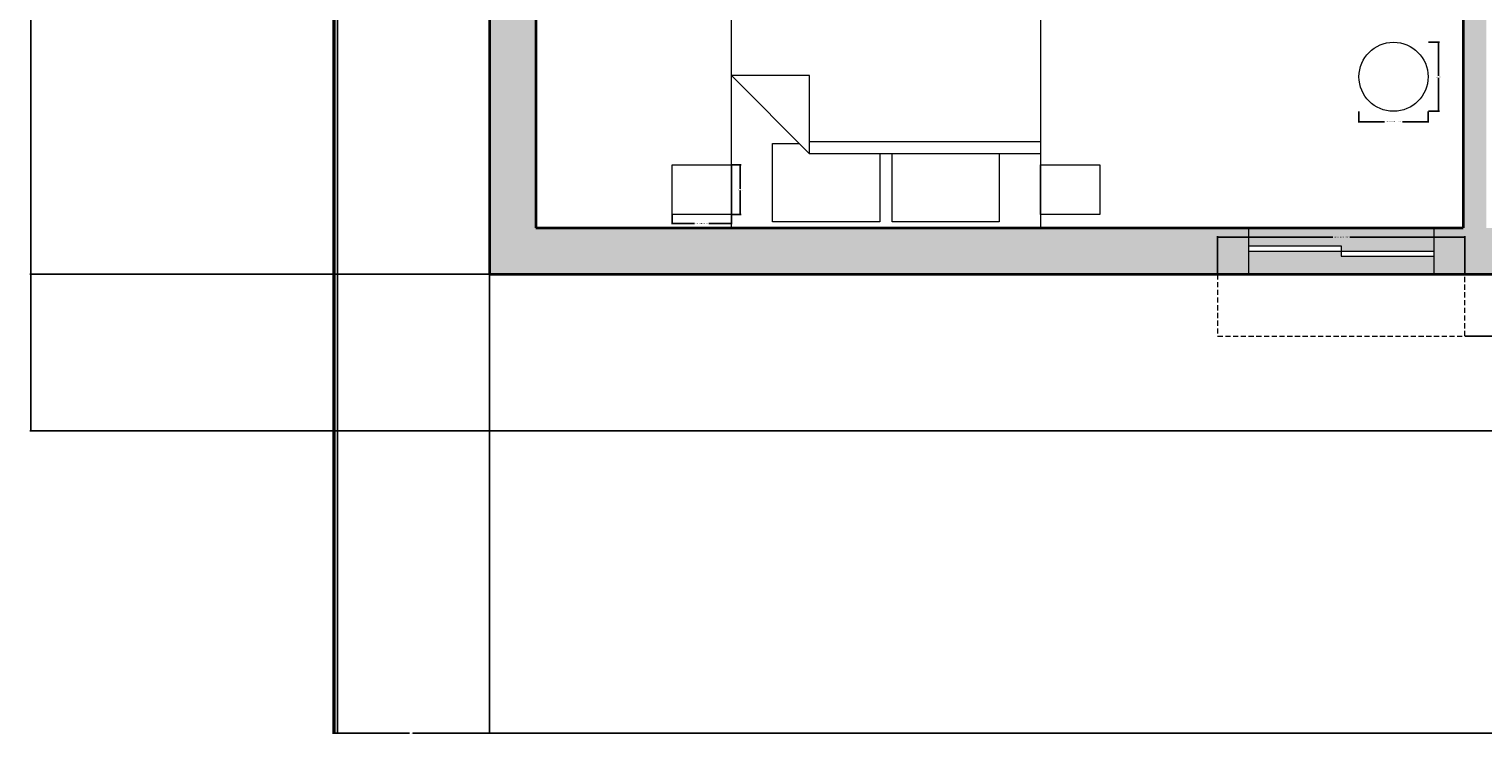
# Model space of a CAD drawing. Units: inches. Extents: x 1693 to 2974, y 2201 to 2965.
# Tile 1 of 24: x 1693 to 1976, y 2201 to 2337. Entities that reach past the tile are written whole.
import ezdxf

# ---------------------------------------------------------------- set-up
doc = ezdxf.new("R2010")
doc.units = ezdxf.units.IN
doc.header["$LTSCALE"] = 2
doc.header["$MEASUREMENT"] = 0
doc.linetypes.add('HIDDEN', pattern=[0.375, 0.25, -0.125])
for name, color, linetype, lineweight in [('A-ANNO-DIMS', 2, 'Continuous', 18), ('A-FURN', 8, 'Continuous', 18), ('A-GLAZ', 4, 'Continuous', 18), ('A-GLAZ-OVHD', 8, 'HIDDEN', 13), ('A-WALL', 7, 'Continuous', 35)]:
    doc.layers.add(name, color=color, linetype=linetype, lineweight=lineweight)
doc.layers.add('A-GLAZ-PATT', color=141, linetype='Continuous', lineweight=13, true_color=0xadddf7)
doc.layers.add('A-WALL-PATT', color=251, linetype='Continuous', lineweight=13, true_color=0x636466)
doc.styles.get("Standard").update_dxf_attribs({"font": 'arial.ttf'})
doc.dimstyles.get("Standard").update_dxf_attribs({"dimtxt": 0.18, "dimasz": 0.18, "dimexe": 0.18, "dimexo": 0.0625, "dimgap": 0.09, "dimtad": 0, "dimtih": 1, "dimtoh": 1, "dimdec": 1, "dimzin": 0, "dimdsep": 46, "dimlunit": 3, "dimtxsty": 'Standard', "dimcen": 0.09, "dimadec": 0, "dimazin": 0, "dimtfac": 1, "dimtdec": 1, "dimtofl": 0, "dimtmove": 0, "dimatfit": 3, "dimfxl": 1, "dimtolj": 1, "dimtzin": 0, "dimarcsym": 0})

# ---------------------------------------------------------------- blocks, each defined once
blk = doc.blocks.new('Bed - Queen')
for p, q in [((0, -80.00003), (0, 0)), ((0, 0), (59.99999, 0)), ((59.99999, 0), (59.99999, -80.00003)), ((7.99999, -1.2), (28.79998, -1.2)), ((7.99999, -14.4), (7.99999, -1.2)), ((28.79998, -1.2), (28.79998, -14.4)), ((31.19999, -1.2), (51.99999, -1.2)), ((31.19999, -14.4), (31.19999, -1.2)), ((51.99999, -1.2), (51.99999, -16.4)), ((0, -14.4), (44.8, -14.4)), ((44.8, -16.8), (0, -16.8)), ((59.99999, -29.6), (44.8, -14.4)), ((44.8, -14.4), (44.8, -29.6)), ((51.99999, -16.4), (46.79936, -16.4)), ((44.8, -29.6), (59.99999, -29.6)), ((59.99999, -80.00003), (0, -80.00003))]:
    blk.add_line(p, q)
blk = doc.blocks.new('NIGHTSTAND')
at = {"ltscale": 2}
blk.add_lwpolyline([(11.51, 0), (0, 0), (0, 9.62), (11.51, 9.62)], close=True, dxfattribs=at)
blk = doc.blocks.new('TABLE-END-ROUND')
at = {"ltscale": 2}
blk.add_circle((6.71, 6.71), 6.71, dxfattribs=at)
blk = doc.blocks.new('WINDOW-HOOD-48IN')
at = {"ltscale": 2}
for p, q in [((12, 48), (0, 48)), ((0, 48), (0, 6)), ((12, 42), (12, 48)), ((0, 6), (0, 0)), ((0, 0), (12, 0))]:
    blk.add_line(p, q, dxfattribs=at)
blk = doc.blocks.new('*D29')
at = {"layer": 'A-ANNO-DIMS', "color": 0, "lineweight": -2, "ltscale": 2, "transparency": 16777216}
for p, q in [((1818.16, 2301.4), (1818.16, 2299.55)), ((1829.67, 2301.4), (1829.67, 2299.55)), ((1818.34, 2299.73), (1822.54, 2299.73)), ((1829.49, 2299.73), (1825.29, 2299.73))]:
    blk.add_line(p, q, dxfattribs=at)
at = {"layer": 'A-ANNO-DIMS', "color": 0, "ltscale": 2, "transparency": 16777216}
for points in [[(1818.34, 2299.76), (1818.34, 2299.7), (1818.16, 2299.73)], [(1829.49, 2299.76), (1829.49, 2299.7), (1829.67, 2299.73)]]:
    blk.add_solid(points, dxfattribs=at)
at = {"layer": 'Defpoints', "color": 0, "ltscale": 2, "transparency": 16777216}
for p in [(1818.16, 2301.46), (1829.67, 2301.46), (1829.67, 2299.73)]:
    blk.add_point(p, dxfattribs=at)
at = {"layer": 'A-ANNO-DIMS', "color": 0, "ltscale": 2, "transparency": 16777216, "insert": (1823.92, 2299.73), "char_height": 0.18, "attachment_point": 5}
blk.add_mtext('\\A1;NIGHTSTAND 12 TYP.', dxfattribs=at)
blk = doc.blocks.new('*D30')
at = {"layer": 'A-ANNO-DIMS', "color": 0, "lineweight": -2, "ltscale": 2, "transparency": 16777216}
for p, q in [((1829.73, 2311.08), (1831.58, 2311.08)), ((1831.4, 2310.9), (1831.4, 2306.45)), ((1831.4, 2301.64), (1831.4, 2306.09)), ((1829.73, 2301.46), (1831.58, 2301.46))]:
    blk.add_line(p, q, dxfattribs=at)
at = {"layer": 'A-ANNO-DIMS', "color": 0, "ltscale": 2, "transparency": 16777216}
for points in [[(1831.37, 2310.9), (1831.43, 2310.9), (1831.4, 2311.08)], [(1831.37, 2301.64), (1831.43, 2301.64), (1831.4, 2301.46)]]:
    blk.add_solid(points, dxfattribs=at)
at = {"layer": 'Defpoints', "color": 0, "ltscale": 2, "transparency": 16777216}
for p in [(1829.67, 2311.08), (1831.4, 2311.08), (1829.67, 2301.46)]:
    blk.add_point(p, dxfattribs=at)
at = {"layer": 'A-ANNO-DIMS', "color": 0, "ltscale": 2, "transparency": 16777216, "insert": (1831.4, 2306.27), "char_height": 0.18, "attachment_point": 5}
blk.add_mtext('\\A1;10 TYP.', dxfattribs=at)
blk = doc.blocks.new('*D51')
at = {"layer": 'A-ANNO-DIMS', "color": 0, "lineweight": -2, "ltscale": 2, "transparency": 16777216}
for p, q in [((1924.08, 2289.91), (1924.08, 2297.22)), ((1924.26, 2297.04), (1946.43, 2297.04)), ((1971.9, 2297.04), (1949.73, 2297.04)), ((1972.08, 2289.91), (1972.08, 2297.22))]:
    blk.add_line(p, q, dxfattribs=at)
at = {"layer": 'A-ANNO-DIMS', "color": 0, "ltscale": 2, "transparency": 16777216}
for points in [[(1924.26, 2297.07), (1924.26, 2297.01), (1924.08, 2297.04)], [(1971.9, 2297.07), (1971.9, 2297.01), (1972.08, 2297.04)]]:
    blk.add_solid(points, dxfattribs=at)
at = {"layer": 'Defpoints', "color": 0, "ltscale": 2, "transparency": 16777216}
for p in [(1924.08, 2297.04), (1924.08, 2289.84), (1972.08, 2289.84)]:
    blk.add_point(p, dxfattribs=at)
at = {"layer": 'A-ANNO-DIMS', "color": 0, "ltscale": 2, "transparency": 16777216, "insert": (1948.08, 2297.04), "char_height": 0.18, "attachment_point": 5}
blk.add_mtext('\\A1;WINDOW HOOD B 48 TYP.', dxfattribs=at)
blk = doc.blocks.new('*D52')
at = {"layer": 'A-ANNO-DIMS', "color": 0, "lineweight": -2, "ltscale": 2, "transparency": 16777216}
for p, q in [((1972.14, 2289.84), (1979.46, 2289.84)), ((1979.28, 2289.66), (1979.28, 2284.03)), ((1979.28, 2278.02), (1979.28, 2283.66)), ((1972.14, 2277.84), (1979.46, 2277.84))]:
    blk.add_line(p, q, dxfattribs=at)
at = {"layer": 'A-ANNO-DIMS', "color": 0, "ltscale": 2, "transparency": 16777216}
for points in [[(1979.25, 2289.66), (1979.31, 2289.66), (1979.28, 2289.84)], [(1979.25, 2278.02), (1979.31, 2278.02), (1979.28, 2277.84)]]:
    blk.add_solid(points, dxfattribs=at)
at = {"layer": 'Defpoints', "color": 0, "ltscale": 2, "transparency": 16777216}
for p in [(1972.08, 2289.84), (1979.28, 2289.84), (1972.08, 2277.84)]:
    blk.add_point(p, dxfattribs=at)
at = {"layer": 'A-ANNO-DIMS', "color": 0, "ltscale": 2, "transparency": 16777216, "insert": (1979.28, 2283.84), "char_height": 0.18, "attachment_point": 5}
blk.add_mtext('\\A1;12 TYP.', dxfattribs=at)
blk = doc.blocks.new('*D75')
at = {"layer": 'A-ANNO-DIMS', "color": 0, "lineweight": -2, "ltscale": 2, "transparency": 16777216}
for p, q in [((1951.51, 2321.44), (1951.51, 2319.31)), ((1964.93, 2321.44), (1964.93, 2319.31)), ((1951.69, 2319.49), (1956.47, 2319.49)), ((1964.75, 2319.49), (1959.98, 2319.49))]:
    blk.add_line(p, q, dxfattribs=at)
at = {"layer": 'A-ANNO-DIMS', "color": 0, "ltscale": 2, "transparency": 16777216}
for points in [[(1951.69, 2319.52), (1951.69, 2319.46), (1951.51, 2319.49)], [(1964.75, 2319.52), (1964.75, 2319.46), (1964.93, 2319.49)]]:
    blk.add_solid(points, dxfattribs=at)
at = {"layer": 'Defpoints', "color": 0, "ltscale": 2, "transparency": 16777216}
for p in [(1951.51, 2321.5), (1964.93, 2321.5), (1964.93, 2319.49)]:
    blk.add_point(p, dxfattribs=at)
at = {"layer": 'A-ANNO-DIMS', "color": 0, "ltscale": 2, "transparency": 16777216, "insert": (1958.22, 2319.49), "char_height": 0.18, "attachment_point": 5}
blk.add_mtext('\\A1;ROUND END TABLE 13 TYP.', dxfattribs=at)
blk = doc.blocks.new('*D76')
at = {"layer": 'A-ANNO-DIMS', "color": 0, "lineweight": -2, "ltscale": 2, "transparency": 16777216}
for p, q in [((1965, 2334.92), (1967.13, 2334.92)), ((1966.95, 2334.74), (1966.95, 2328.4)), ((1966.95, 2321.68), (1966.95, 2328.03)), ((1965, 2321.5), (1967.13, 2321.5))]:
    blk.add_line(p, q, dxfattribs=at)
at = {"layer": 'A-ANNO-DIMS', "color": 0, "ltscale": 2, "transparency": 16777216}
for points in [[(1966.92, 2334.74), (1966.98, 2334.74), (1966.95, 2334.92)], [(1966.92, 2321.68), (1966.98, 2321.68), (1966.95, 2321.5)]]:
    blk.add_solid(points, dxfattribs=at)
at = {"layer": 'Defpoints', "color": 0, "ltscale": 2, "transparency": 16777216}
for p in [(1964.93, 2334.92), (1966.95, 2334.92), (1964.93, 2321.5)]:
    blk.add_point(p, dxfattribs=at)
at = {"layer": 'A-ANNO-DIMS', "color": 0, "ltscale": 2, "transparency": 16777216, "insert": (1966.95, 2328.21), "char_height": 0.18, "attachment_point": 5}
blk.add_mtext('\\A1;13 TYP.', dxfattribs=at)
blk = doc.blocks.new('*D82')
at = {"layer": 'A-ANNO-DIMS', "color": 0, "lineweight": -2, "ltscale": 2, "transparency": 16777216}
for p, q in [((2615.67, 2906.08), (1693.46, 2906.08)), ((1693.64, 2905.9), (1693.64, 2582.94)), ((1693.64, 2259.62), (1693.64, 2582.58)), ((2096.17, 2259.44), (1693.46, 2259.44))]:
    blk.add_line(p, q, dxfattribs=at)
at = {"layer": 'A-ANNO-DIMS', "color": 0, "ltscale": 2, "transparency": 16777216}
for points in [[(1693.61, 2905.9), (1693.67, 2905.9), (1693.64, 2906.08)], [(1693.61, 2259.62), (1693.67, 2259.62), (1693.64, 2259.44)]]:
    blk.add_solid(points, dxfattribs=at)
at = {"layer": 'Defpoints', "color": 0, "ltscale": 2, "transparency": 16777216}
for p in [(1693.64, 2906.08), (2615.74, 2906.08), (2096.24, 2259.44)]:
    blk.add_point(p, dxfattribs=at)
at = {"layer": 'A-ANNO-DIMS', "color": 0, "ltscale": 2, "transparency": 16777216, "insert": (1693.64, 2582.76), "char_height": 0.18, "attachment_point": 5}
blk.add_mtext('\\A1;646.6', dxfattribs=at)
blk = doc.blocks.new('*D83')
at = {"layer": 'A-ANNO-DIMS', "color": 0, "lineweight": -2, "ltscale": 2, "transparency": 16777216}
for p, q in [((1782.74, 2289.78), (1782.74, 2200.56)), ((2294.24, 2289.78), (2294.24, 2200.56)), ((1782.92, 2200.74), (2038.09, 2200.74)), ((2294.06, 2200.74), (2038.88, 2200.74))]:
    blk.add_line(p, q, dxfattribs=at)
at = {"layer": 'A-ANNO-DIMS', "color": 0, "ltscale": 2, "transparency": 16777216}
for points in [[(1782.92, 2200.77), (1782.92, 2200.71), (1782.74, 2200.74)], [(2294.06, 2200.77), (2294.06, 2200.71), (2294.24, 2200.74)]]:
    blk.add_solid(points, dxfattribs=at)
at = {"layer": 'Defpoints', "color": 0, "ltscale": 2, "transparency": 16777216}
for p in [(1782.74, 2289.84), (2294.24, 2289.84), (2294.24, 2200.74)]:
    blk.add_point(p, dxfattribs=at)
at = {"layer": 'A-ANNO-DIMS', "color": 0, "ltscale": 2, "transparency": 16777216, "insert": (2038.49, 2200.74), "char_height": 0.18, "attachment_point": 5}
blk.add_mtext('\\A1;511.5', dxfattribs=at)
blk = doc.blocks.new('*D86')
at = {"layer": 'A-ANNO-DIMS', "color": 0, "lineweight": -2, "ltscale": 2, "transparency": 16777216}
for p, q in [((1782.67, 2706.84), (1693.46, 2706.84)), ((1693.64, 2706.66), (1693.64, 2498.53)), ((1693.64, 2290.02), (1693.64, 2498.16)), ((1782.67, 2289.84), (1693.46, 2289.84))]:
    blk.add_line(p, q, dxfattribs=at)
at = {"layer": 'A-ANNO-DIMS', "color": 0, "ltscale": 2, "transparency": 16777216}
for points in [[(1693.61, 2706.66), (1693.67, 2706.66), (1693.64, 2706.84)], [(1693.61, 2290.02), (1693.67, 2290.02), (1693.64, 2289.84)]]:
    blk.add_solid(points, dxfattribs=at)
at = {"layer": 'Defpoints', "color": 0, "ltscale": 2, "transparency": 16777216}
for p in [(1693.64, 2706.84), (1782.74, 2706.84), (1782.74, 2289.84)]:
    blk.add_point(p, dxfattribs=at)
at = {"layer": 'A-ANNO-DIMS', "color": 0, "ltscale": 2, "transparency": 16777216, "insert": (1693.64, 2498.34), "char_height": 0.18, "attachment_point": 5}
blk.add_mtext('\\A1;417', dxfattribs=at)
blk = doc.blocks.new('*D92')
at = {"layer": 'A-ANNO-DIMS', "color": 0, "lineweight": -2, "ltscale": 2, "transparency": 16777216}
for p, q in [((1752.34, 2442.78), (1752.34, 2200.56)), ((1782.74, 2442.78), (1782.74, 2200.56)), ((1752.52, 2200.74), (1767.21, 2200.74)), ((1782.56, 2200.74), (1767.86, 2200.74))]:
    blk.add_line(p, q, dxfattribs=at)
at = {"layer": 'A-ANNO-DIMS', "color": 0, "ltscale": 2, "transparency": 16777216}
for points in [[(1752.52, 2200.77), (1752.52, 2200.71), (1752.34, 2200.74)], [(1782.56, 2200.77), (1782.56, 2200.71), (1782.74, 2200.74)]]:
    blk.add_solid(points, dxfattribs=at)
at = {"layer": 'Defpoints', "color": 0, "ltscale": 2, "transparency": 16777216}
for p in [(1752.34, 2442.84), (1782.74, 2442.84), (1782.74, 2200.74)]:
    blk.add_point(p, dxfattribs=at)
at = {"layer": 'A-ANNO-DIMS', "color": 0, "ltscale": 2, "transparency": 16777216, "insert": (1767.54, 2200.74), "char_height": 0.18, "attachment_point": 5}
blk.add_mtext('\\A1;30.4', dxfattribs=at)
blk = doc.blocks.new('*D107')
at = {"layer": 'A-ANNO-DIMS', "color": 0, "lineweight": -2, "ltscale": 2, "transparency": 16777216}
for p, q in [((1752.68, 2456.67), (1752.68, 2200.56)), ((1753.22, 2456.67), (1753.22, 2200.56)), ((1752.86, 2200.74), (1753.04, 2200.74)), ((1753.22, 2200.74), (1753.4, 2200.74))]:
    blk.add_line(p, q, dxfattribs=at)
at = {"layer": 'A-ANNO-DIMS', "color": 0, "ltscale": 2, "transparency": 16777216}
for points in [[(1752.86, 2200.77), (1752.86, 2200.71), (1752.68, 2200.74)], [(1753.04, 2200.77), (1753.04, 2200.71), (1753.22, 2200.74)]]:
    blk.add_solid(points, dxfattribs=at)
at = {"layer": 'Defpoints', "color": 0, "ltscale": 2, "transparency": 16777216}
for p in [(1752.68, 2456.73), (1753.22, 2456.73), (1753.22, 2200.74)]:
    blk.add_point(p, dxfattribs=at)
at = {"layer": 'A-ANNO-DIMS', "color": 0, "ltscale": 2, "transparency": 16777216, "insert": (1753.8, 2200.74), "char_height": 0.18, "attachment_point": 5}
blk.add_mtext('\\A1;0.547', dxfattribs=at)

msp = doc.modelspace()

# ---------------------------------------------------------------- hatches: boundary and pattern name
at = {"layer": 'A-GLAZ-PATT', "ltscale": 2}
h = msp.add_hatch(color=256, dxfattribs=at)
h.dxf.hatch_style = 1
h.paths.add_polyline_path([(2656.9702, 2338.2547), (2632.9702, 2338.2547), (2632.9702, 2339.2547), (2608.9702, 2339.2547), (2608.9702, 2334.7547), (2656.9702, 2334.7547)])
h.paths.add_polyline_path([(2656.9702, 2343.7547), (2608.9702, 2343.7547), (2608.9702, 2340.2547), (2632.9702, 2340.2547), (2632.9702, 2339.2547), (2656.9702, 2339.2547)])
h.paths.add_polyline_path([(2775.7544, 2338.2547), (2751.7544, 2338.2547), (2751.7544, 2334.7547), (2775.7544, 2334.7547)])
h.paths.add_polyline_path([(2775.7544, 2343.7547), (2751.7544, 2343.7547), (2751.7544, 2340.2547), (2775.7544, 2340.2547)])
h.paths.add_polyline_path([(2897.7363, 2568.7999), (2893.2363, 2568.7999), (2893.2363, 2520.7999), (2896.7363, 2520.7999), (2896.7363, 2544.7999), (2897.7363, 2544.7999)])
h.paths.add_polyline_path([(2902.2363, 2568.7999), (2898.7363, 2568.7999), (2898.7363, 2544.7999), (2897.7363, 2544.7999), (2897.7363, 2520.7999), (2902.2363, 2520.7999)])
h.paths.add_polyline_path([(2902.2363, 2637.7547), (2898.7363, 2637.7547), (2898.7363, 2613.7547), (2902.2363, 2613.7547)])
h.paths.add_polyline_path([(2896.7363, 2637.7547), (2893.2363, 2637.7547), (2893.2363, 2613.7547), (2896.7363, 2613.7547)])
h.paths.add_polyline_path([(2902.2363, 2748.903), (2899.0477, 2748.903), (2899.0477, 2724.903), (2898.0477, 2724.903), (2898.0477, 2700.903), (2902.2363, 2700.903)])
h.paths.add_polyline_path([(2898.0477, 2748.903), (2893.2363, 2748.903), (2893.2363, 2700.903), (2897.0477, 2700.903), (2897.0477, 2724.903), (2898.0477, 2724.903)])
h.paths.add_polyline_path([(2851.2363, 2846.2547), (2803.2363, 2846.2547), (2803.2363, 2842.7547), (2827.2363, 2842.7547), (2827.2363, 2841.7547), (2851.2363, 2841.7547)])
h.paths.add_polyline_path([(2851.2363, 2840.7547), (2827.2363, 2840.7547), (2827.2363, 2841.7547), (2803.2363, 2841.7547), (2803.2363, 2837.2547), (2851.2363, 2837.2547)])
h.paths.add_polyline_path([(2578.2363, 2846.2547), (2530.2363, 2846.2547), (2530.2363, 2842.7547), (2554.2363, 2842.7547), (2554.2363, 2841.7547), (2578.2363, 2841.7547)])
h.paths.add_polyline_path([(2578.2363, 2840.7547), (2554.2363, 2840.7547), (2554.2363, 2841.7547), (2530.2363, 2841.7547), (2530.2363, 2837.2547), (2578.2363, 2837.2547)])
h.paths.add_polyline_path([(2732.7363, 2812.7547), (2705.1363, 2812.7547), (2705.1363, 2811.7547), (2676.3363, 2811.7547), (2676.3363, 2812.7547), (2648.7363, 2812.7547), (2648.7363, 2808.2547), (2732.7363, 2808.2547)])
h.paths.add_polyline_path([(2732.7363, 2817.2547), (2648.7363, 2817.2547), (2648.7363, 2813.7547), (2676.3363, 2813.7547), (2676.3363, 2812.7547), (2705.1363, 2812.7547), (2705.1363, 2813.7547), (2732.7363, 2813.7547)])
h.paths.add_polyline_path([(2488.2363, 2695.8203), (2484.7878, 2695.8203), (2484.7878, 2671.8203), (2488.2363, 2671.8203)])
h.paths.add_polyline_path([(2482.7878, 2695.8203), (2479.2363, 2695.8203), (2479.2363, 2671.8203), (2482.7878, 2671.8203)])
h.paths.add_polyline_path([(2488.2363, 2572.4371), (2484.7363, 2572.4371), (2484.7363, 2541.4371), (2483.7363, 2541.4371), (2483.7363, 2512.4371), (2488.2363, 2512.4371)])
h.paths.add_polyline_path([(2482.7363, 2541.4371), (2483.7363, 2541.4371), (2483.7363, 2572.4371), (2479.2363, 2572.4371), (2479.2363, 2512.4371), (2482.7363, 2512.4371)])
h.paths.add_polyline_path([(2248.9863, 2706.8449), (2190.9863, 2706.8449), (2190.9863, 2703.3449), (2219.9863, 2703.3449), (2219.9863, 2702.3449), (2248.9863, 2702.3449)])
h.paths.add_polyline_path([(2248.9863, 2701.3449), (2219.9863, 2701.3449), (2219.9863, 2702.3449), (2190.9863, 2702.3449), (2190.9863, 2697.8449), (2248.9863, 2697.8449)])
h.paths.add_polyline_path([(2151.9207, 2293.3449), (2127.9207, 2293.3449), (2127.9207, 2289.8449), (2151.9207, 2289.8449)])
h.paths.add_polyline_path([(2151.9207, 2298.8449), (2127.9207, 2298.8449), (2127.9207, 2295.3449), (2151.9207, 2295.3449)])
h.paths.add_polyline_path([(2084.023, 2293.3449), (2066.023, 2293.3449), (2066.023, 2294.3449), (2048.023, 2294.3449), (2048.023, 2289.8449), (2084.023, 2289.8449)])
h.paths.add_polyline_path([(2084.023, 2298.8449), (2048.023, 2298.8449), (2048.023, 2295.3449), (2066.023, 2295.3449), (2066.023, 2294.3449), (2084.023, 2294.3449)])
h.paths.add_polyline_path([(1966.0781, 2293.3449), (1948.0781, 2293.3449), (1948.0781, 2294.3449), (1930.0781, 2294.3449), (1930.0781, 2289.8449), (1966.0781, 2289.8449)])
h.paths.add_polyline_path([(1966.0781, 2298.8449), (1930.0781, 2298.8449), (1930.0781, 2295.3449), (1948.0781, 2295.3449), (1948.0781, 2294.3449), (1966.0781, 2294.3449)])
h.paths.add_polyline_path([(1787.2363, 2403.1922), (1782.7363, 2403.1922), (1782.7363, 2355.1922), (1786.2363, 2355.1922), (1786.2363, 2379.1922), (1787.2363, 2379.1922)])
h.paths.add_polyline_path([(1791.7363, 2403.1922), (1788.2363, 2403.1922), (1788.2363, 2379.1922), (1787.2363, 2379.1922), (1787.2363, 2355.1922), (1791.7363, 2355.1922)])
h.paths.add_polyline_path([(1786.2363, 2477.5455), (1782.7363, 2477.5455), (1782.7363, 2453.5455), (1786.2363, 2453.5455)])
h.paths.add_polyline_path([(1791.7363, 2477.5455), (1788.2363, 2477.5455), (1788.2363, 2453.5455), (1791.7363, 2453.5455)])
h.paths.add_polyline_path([(1786.2363, 2621.6433), (1782.7363, 2621.6433), (1782.7363, 2585.6433), (1786.2363, 2585.6433)])
h.paths.add_polyline_path([(1791.7363, 2621.6433), (1788.2363, 2621.6433), (1788.2363, 2585.6433), (1791.7363, 2585.6433)])
h.paths.add_polyline_path([(1908.1286, 2706.8449), (1860.1286, 2706.8449), (1860.1286, 2703.3449), (1884.1286, 2703.3449), (1884.1286, 2702.3449), (1908.1286, 2702.3449)])
h.paths.add_polyline_path([(1908.1286, 2701.3449), (1884.1286, 2701.3449), (1884.1286, 2702.3449), (1860.1286, 2702.3449), (1860.1286, 2697.8449), (1908.1286, 2697.8449)])
h.paths.add_polyline_path([(1973.9863, 2706.8449), (1949.9863, 2706.8449), (1949.9863, 2703.3449), (1973.9863, 2703.3449)])
h.paths.add_polyline_path([(1973.9863, 2701.3449), (1949.9863, 2701.3449), (1949.9863, 2697.8449), (1973.9863, 2697.8449)])
h.paths.add_polyline_path([(2112.7363, 2690.3449), (2028.7363, 2690.3449), (2028.7363, 2686.8449), (2056.3363, 2686.8449), (2056.3363, 2685.8449), (2085.1363, 2685.8449), (2085.1363, 2686.8449), (2112.7363, 2686.8449)])
h.paths.add_polyline_path([(2112.7363, 2685.8449), (2085.1363, 2685.8449), (2085.1363, 2684.8449), (2056.3363, 2684.8449), (2056.3363, 2685.8449), (2028.7363, 2685.8449), (2028.7363, 2681.3449), (2112.7363, 2681.3449)])
h.paths.add_polyline_path([(2422.7363, 2640.7547), (2350.7363, 2640.7547), (2350.7363, 2637.2547), (2386.7363, 2637.2547), (2386.7363, 2636.2547), (2422.7363, 2636.2547)])
h.paths.add_polyline_path([(2422.7363, 2635.2547), (2386.7363, 2635.2547), (2386.7363, 2636.2547), (2350.7363, 2636.2547), (2350.7363, 2631.7547), (2422.7363, 2631.7547)])
at = {"layer": 'A-WALL-PATT', "ltscale": 2}
h = msp.add_hatch(color=256, dxfattribs=at)
h.dxf.hatch_style = 1
h.paths.add_polyline_path([(1928.2363, 2733.2161), (1930.9384, 2733.2161), (1930.9384, 2737.2161), (1923.7363, 2737.2161), (1923.7363, 2706.8449), (1908.1286, 2706.8449), (1908.1286, 2697.8449), (1923.7363, 2697.8449), (1923.7363, 2692.8449), (1928.2363, 2692.8449), (1928.2363, 2697.8449), (1949.9863, 2697.8449), (1949.9863, 2706.8449), (1928.2363, 2706.8449)])
h.paths.add_polyline_path([(2004.7363, 2737.2161), (1995.7363, 2737.2161), (1995.7363, 2706.8449), (1985.6374, 2706.8449), (1973.9863, 2706.8449), (1973.9863, 2697.8449), (2000.2363, 2697.8449), (2000.2363, 2686.5348), (2000.3613, 2686.5348), (2000.3613, 2667.0432), (2000.2363, 2601.8449), (1928.2363, 2601.8449), (1928.2363, 2662.8449), (1923.7363, 2662.8449), (1923.7363, 2595.3449), (1928.2363, 2595.3449), (1928.2363, 2597.3449), (2004.7363, 2597.3449), (2004.7363, 2681.3449), (2012.7814, 2681.3449), (2028.7363, 2681.3449), (2028.7363, 2690.3449), (2004.7363, 2690.3449)])
h.paths.add_polyline_path([(2190.9863, 2706.8449), (2184.9863, 2706.8449), (2145.7363, 2706.8449), (2145.7363, 2765.3449), (2145.7363, 2774.5394), (2136.7363, 2774.5394), (2136.7363, 2756.3449), (2136.7363, 2690.3449), (2112.7363, 2690.3449), (2112.7363, 2681.3449), (2136.7363, 2681.3449), (2136.7363, 2597.3449), (2141.2363, 2597.3449), (2141.2363, 2697.8449), (2190.9863, 2697.8449)])
h.paths.add_polyline_path([(1860.1286, 2706.8449), (1782.7363, 2706.8449), (1782.7363, 2621.6433), (1791.7363, 2621.6433), (1791.7363, 2697.8449), (1860.1286, 2697.8449)])
h.paths.add_polyline_path([(1791.7363, 2585.6433), (1782.7363, 2585.6433), (1782.7363, 2562.8449), (1782.7363, 2553.8449), (1752.3363, 2553.8449), (1752.3363, 2544.2586), (1756.3363, 2544.2586), (1756.3363, 2549.3449), (1782.7363, 2549.3449), (1782.7363, 2489.2404), (1782.7363, 2477.5455), (1791.7363, 2477.5455), (1791.7363, 2493.5991), (1791.6113, 2493.5991), (1791.6113, 2513.0907), (1791.6824, 2533.7198, -0.94742783), (1791.7363, 2534.7168), (1791.7363, 2549.3449), (1863.7363, 2549.3449), (1863.7363, 2513.3449), (1866.7363, 2513.3449), (1866.7363, 2549.3449), (1924.7363, 2549.3449), (1924.7363, 2447.3449), (1924.7363, 2442.8449), (1933.7363, 2442.8449), (1933.7363, 2447.3449), (1928.2363, 2447.3449), (1928.2363, 2559.3449), (1923.7363, 2559.3449), (1923.7363, 2553.8449), (1791.7363, 2553.8449), (1791.7363, 2562.8449)])
h.paths.add_polyline_path([(1791.7363, 2442.8449), (1866.7363, 2442.8449), (1866.7363, 2447.3449), (1866.7363, 2483.3449), (1863.7363, 2483.3449), (1863.7363, 2447.3449), (1791.7363, 2447.3449), (1791.7363, 2453.5455), (1782.7363, 2453.5455), (1782.7363, 2447.3449), (1756.3363, 2447.3449), (1756.3363, 2455.7126), (1752.3363, 2455.7126), (1752.3363, 2442.8449), (1782.7363, 2442.8449), (1782.7363, 2403.1922), (1791.7363, 2403.1922)])
h.paths.add_polyline_path([(1930.0781, 2298.8449), (1791.7363, 2298.8449), (1791.7363, 2355.1922), (1782.7363, 2355.1922), (1782.7363, 2289.8449), (1930.0781, 2289.8449)])
h.paths.add_polyline_path([(2624.7363, 2883.2547), (2624.7363, 2902.6165), (2624.7363, 2906.0761), (2615.7363, 2906.0761), (2615.7363, 2892.2547), (2615.7363, 2846.2547), (2578.2363, 2846.2547), (2578.2363, 2837.2547), (2620.2363, 2837.2547), (2620.2363, 2743.2547), (2624.7363, 2743.2547), (2624.7363, 2808.2547), (2648.7363, 2808.2547), (2648.7363, 2817.2547), (2624.7363, 2817.2547)])
h.paths.add_polyline_path([(2530.2363, 2846.2547), (2479.2363, 2846.2547), (2479.2363, 2695.8203), (2488.2363, 2695.8203), (2488.2363, 2700.7547), (2567.2363, 2700.7547), (2567.2363, 2705.2547), (2488.2363, 2705.2547), (2488.2363, 2837.2547), (2530.2363, 2837.2547)])
h.paths.add_polyline_path([(2488.2363, 2487.7547), (2630.2363, 2487.7547, -0.00990191), (2630.2363, 2489.0322), (2630.2363, 2492.2547), (2488.2363, 2492.2547), (2488.2363, 2512.4371), (2479.2363, 2512.4371), (2479.2363, 2334.7547), (2608.9702, 2334.7547), (2608.9702, 2343.7547), (2488.2363, 2343.7547)])
h.paths.add_polyline_path([(2751.7544, 2343.7547), (2672.7363, 2343.7547), (2672.7363, 2409.7547), (2674.7363, 2409.7547), (2674.7363, 2413.7547), (2672.7363, 2413.7547), (2672.7363, 2487.7547), (2732.7363, 2487.7547), (2732.7363, 2413.7547), (2704.7363, 2413.7547), (2704.7363, 2409.7547), (2784.7363, 2409.7547), (2784.7363, 2343.7547), (2775.7544, 2343.7547), (2775.7544, 2334.7547), (2902.2363, 2334.7547), (2902.2363, 2520.7999), (2893.2363, 2520.7999), (2893.2363, 2413.7547), (2856.0145, 2413.7547), (2856.0145, 2409.7547), (2893.2363, 2409.7547), (2893.2363, 2343.7547), (2789.2363, 2343.7547), (2789.2363, 2409.7547), (2819.2363, 2409.7547), (2826.0145, 2409.7547), (2826.0145, 2413.7547), (2789.2363, 2413.7547), (2789.2363, 2492.2547), (2784.7363, 2492.2547), (2784.7363, 2413.7547), (2736.7363, 2413.7547), (2736.7363, 2492.2547), (2672.7363, 2492.2547), (2666.2363, 2492.2547), (2666.2363, 2487.7547), (2668.2363, 2487.7547), (2668.2363, 2343.7547), (2656.9702, 2343.7547), (2656.9702, 2334.7547), (2662.9702, 2334.7547), (2751.7544, 2334.7547)])
h.paths.add_polyline_path([(2902.2363, 2613.7547), (2893.2363, 2613.7547), (2893.2363, 2589.7547), (2785.2363, 2589.7547), (2785.2363, 2661.7547), (2790.2363, 2661.7547), (2790.2363, 2665.2547), (2761.2363, 2665.2547), (2761.2363, 2667.2547), (2756.7363, 2667.2547), (2756.7363, 2661.7547), (2781.2363, 2661.7547), (2781.2363, 2585.7547), (2893.2363, 2585.7547), (2893.2363, 2568.7999), (2902.2363, 2568.7999)])
h.paths.add_polyline_path([(2488.2363, 2671.8203), (2479.2363, 2671.8203), (2479.2363, 2645.2547), (2479.2363, 2623.4598), (2488.2363, 2623.4598), (2488.2363, 2636.2547), (2624.7363, 2636.2547), (2624.7363, 2640.7547), (2603.7363, 2640.7547), (2603.7363, 2700.7547), (2624.7363, 2700.7547), (2624.7363, 2707.2547), (2620.2363, 2707.2547), (2620.2363, 2705.2547), (2597.2363, 2705.2547), (2597.2363, 2700.7547), (2599.2363, 2700.7547), (2599.2363, 2640.7547), (2488.2363, 2640.7547)])
h.paths.add_polyline_path([(2761.2363, 2837.2547), (2803.2363, 2837.2547), (2803.2363, 2846.2547), (2797.2363, 2846.2547), (2765.7363, 2846.2547), (2756.7363, 2846.2547), (2756.7363, 2817.2547), (2732.7363, 2817.2547), (2732.7363, 2808.2547), (2756.7363, 2808.2547), (2756.7363, 2703.2547), (2761.2363, 2703.2547)])
h.paths.add_polyline_path([(2739.7489, 2433.1234), (2786.9181, 2433.1234), (2786.9181, 2455.5122), (2739.7489, 2455.5122)], flags=25)
h = msp.add_hatch(color=256, dxfattribs=at)
h.dxf.hatch_style = 1
h.paths.add_polyline_path([(2294.2363, 2706.8449), (2248.9863, 2706.8449), (2248.9863, 2697.8449), (2285.2363, 2697.8449), (2285.2363, 2586.2648), (2294.2363, 2586.2648)])
h.paths.add_polyline_path([(2294.2363, 2550.2648), (2285.2363, 2550.2648), (2285.2363, 2517.8449), (2141.2363, 2517.8449), (2141.2363, 2513.8449), (2285.2363, 2513.8449), (2285.2363, 2369.8449), (2253.0704, 2369.8449), (2253.0704, 2366.8449), (2285.2363, 2366.8449), (2285.2363, 2298.8449), (2165.2363, 2298.8449), (2165.2363, 2366.8449), (2165.2363, 2369.8449), (2165.2363, 2447.3449), (2160.7363, 2447.3449), (2160.7363, 2403.3449), (2100.7363, 2403.3449), (2100.7363, 2447.3449), (2094.2363, 2447.3449), (2094.2363, 2442.8449), (2096.2363, 2442.8449), (2096.2363, 2362.1344), (2100.7363, 2362.1344), (2100.7363, 2400.8449), (2160.7363, 2400.8449), (2160.7363, 2298.8449), (2151.9207, 2298.8449), (2151.9207, 2289.8449), (2184.7363, 2289.8449), (2184.7363, 2276.6449), (2189.2363, 2276.6449), (2189.2363, 2289.8449), (2294.2363, 2289.8449)])
h.paths.add_polyline_path([(2048.023, 2298.8449), (1976.2363, 2298.8449), (1976.2363, 2442.8449), (2058.2363, 2442.8449, -0.00822734), (2058.2363, 2443.9061), (2058.2363, 2447.3449), (2004.7363, 2447.3449), (1969.7363, 2447.3449), (1969.7363, 2442.8449), (1971.7363, 2442.8449), (1971.7363, 2298.8449), (1966.0781, 2298.8449), (1966.0781, 2289.8449), (2048.023, 2289.8449)])
h.paths.add_polyline_path([(2127.9207, 2298.8449), (2100.7363, 2298.8449), (2100.7363, 2332.1344), (2096.2363, 2332.1344), (2096.2363, 2298.8449), (2084.023, 2298.8449), (2084.023, 2289.8449), (2096.2363, 2289.8449), (2096.2363, 2259.4449), (2114.3201, 2259.4449), (2114.3201, 2263.4449), (2100.7363, 2263.4449), (2100.7363, 2289.8449), (2127.9207, 2289.8449)])

# ---------------------------------------------------------------- linework, layer by layer
at = {"layer": 'A-GLAZ', "ltscale": 2}
for p, q in [((1930.0781, 2298.8449), (1930.0781, 2289.8449)), ((1966.0781, 2298.8449), (1966.0781, 2289.8449)), ((1930.0781, 2295.3449), (1948.0781, 2295.3449)), ((1948.0781, 2295.3449), (1948.0781, 2293.3449)), ((1930.0781, 2294.3449), (1966.0781, 2294.3449)), ((1948.0781, 2293.3449), (1966.0781, 2293.3449))]:
    msp.add_line(p, q, dxfattribs=at)
at = {"layer": 'A-WALL'}
for p, q in [((1782.7363, 2442.8449), (1782.7363, 2289.8449)), ((1791.7363, 2442.8449), (1791.7363, 2298.8449)), ((1971.7363, 2442.8449), (1971.7363, 2298.8449)), ((1791.7363, 2298.8449), (1971.7363, 2298.8449)), ((1782.7363, 2289.8449), (2096.2363, 2289.8449))]:
    msp.add_line(p, q, dxfattribs=at)

# ---------------------------------------------------------------- block references
at = {"layer": 'A-FURN', "ltscale": 2, "rotation": 180}
msp.add_blockref('Bed - Queen', (1889.6709, 2298.8449), dxfattribs=at)
at = {"layer": 'A-FURN'}
for name, p in [('TABLE-END-ROUND', (1951.513, 2321.503)), ('NIGHTSTAND', (1818.161, 2301.459)), ('NIGHTSTAND', (1889.6708, 2301.459))]:
    msp.add_blockref(name, p, dxfattribs=at)
at = {"layer": 'A-GLAZ-OVHD', "rotation": 90.00000000000044}
msp.add_blockref('WINDOW-HOOD-48IN', (1972.0785, 2277.8446), dxfattribs=at)

# ---------------------------------------------------------------- dimensions: what is measured, and where the dimension line sits
at = {"layer": 'A-ANNO-DIMS', "ltscale": 2}
for base, p1, p2, override, picture, middle in [((1693.6363, 2906.0761), (2096.2363, 2259.4449), (2615.7363, 2906.0761), {"dimdec": 1, "dimlfac": 1, "dimrnd": 0, "dimzin": 0, "dimdsep": 46, "dimlunit": 2}, '*D82', (1693.6363, 2582.7605)), ((1693.6363, 2706.8449), (1782.7363, 2289.8449), (1782.7363, 2706.8449), {"dimdec": 0, "dimlfac": 1, "dimrnd": 0, "dimzin": 0, "dimdsep": 46, "dimlunit": 2}, '*D86', (1693.6363, 2498.3449))]:
    dim = msp.add_linear_dim(base=base, p1=p1, p2=p2, angle=90, dimstyle='Standard', override=override, dxfattribs=at)
    dim.commit()
    dim.dimension.update_dxf_attribs({"geometry": picture, "text_midpoint": middle})
for base, p1, p2, override, picture, middle in [((1753.2225, 2200.7449), (1752.6754, 2456.7302), (1753.2225, 2456.7302), {"dimdec": 3, "dimlfac": 1, "dimrnd": 0, "dimzin": 0, "dimdsep": 46, "dimlunit": 2}, '*D107', (1753.7962, 2200.7449)), ((1782.7363, 2200.7449), (1752.3363, 2442.8449), (1782.7363, 2442.8449), {"dimdec": 1, "dimlfac": 1, "dimrnd": 0, "dimzin": 0, "dimdsep": 46, "dimlunit": 2}, '*D92', (1767.5363, 2200.7449)), ((2294.2363, 2200.7449), (1782.7363, 2289.8449), (2294.2363, 2289.8449), {"dimdec": 1, "dimlfac": 1, "dimrnd": 0, "dimzin": 0, "dimdsep": 46, "dimlunit": 2}, '*D83', (2038.4863, 2200.7449))]:
    dim = msp.add_linear_dim(base=base, p1=p1, p2=p2, dimstyle='Standard', override=override, dxfattribs=at)
    dim.commit()
    dim.dimension.update_dxf_attribs({"geometry": picture, "text_midpoint": middle})
for base, p1, p2, angle, text, picture, middle in [((1966.9473, 2334.9243), (1964.9341, 2321.5033), (1964.9341, 2334.9243), 90, '<> TYP.', '*D76', (1966.9473, 2328.2138)), ((1831.3973, 2311.0775), (1829.6709, 2301.4593), (1829.6709, 2311.0775), 90, '<> TYP.', '*D30', (1831.3973, 2306.2684)), ((1924.0781, 2297.0449), (1972.0781, 2289.8449), (1924.0781, 2289.8449), 180, 'WINDOW HOOD B <> TYP.', '*D51', (1948.0781, 2297.0449)), ((1979.2781, 2289.8449), (1972.0781, 2277.8449), (1972.0781, 2289.8449), 90, '<> TYP.', '*D52', (1979.2781, 2283.8449))]:
    dim = msp.add_linear_dim(base=base, p1=p1, p2=p2, angle=angle, text=text, dimstyle='Standard', override={"dimdec": 0, "dimlfac": 1, "dimrnd": 0, "dimzin": 0, "dimdsep": 46, "dimlunit": 2}, dxfattribs=at)
    dim.commit()
    dim.dimension.update_dxf_attribs({"geometry": picture, "text_midpoint": middle})
for base, p1, p2, text, picture, middle in [((1964.9341, 2319.4901), (1951.5131, 2321.5033), (1964.9341, 2321.5033), 'ROUND END TABLE <> TYP.', '*D75', (1958.2236, 2319.4901)), ((1829.6709, 2299.7328), (1818.161, 2301.4593), (1829.6709, 2301.4593), 'NIGHTSTAND <> TYP.', '*D29', (1823.9159, 2299.7328))]:
    dim = msp.add_linear_dim(base=base, p1=p1, p2=p2, text=text, dimstyle='Standard', override={"dimdec": 0, "dimlfac": 1, "dimrnd": 0, "dimzin": 0, "dimdsep": 46, "dimlunit": 2}, dxfattribs=at)
    dim.commit()
    dim.dimension.update_dxf_attribs({"geometry": picture, "text_midpoint": middle})

doc.saveas('drawing.dxf')
